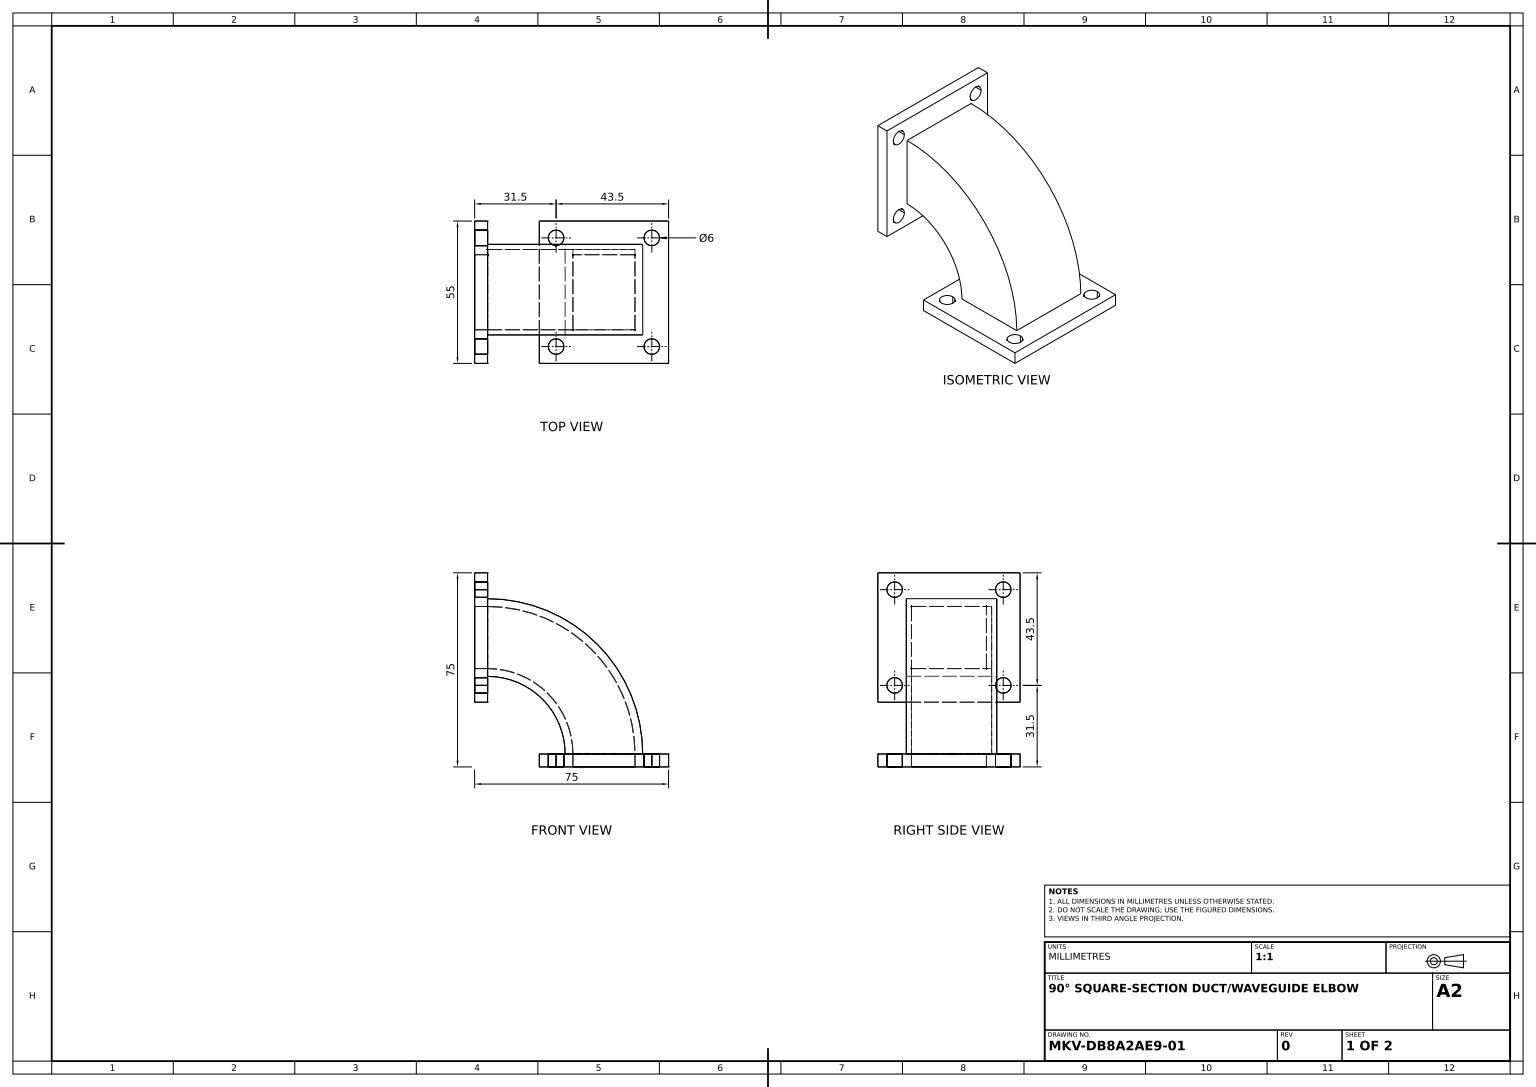
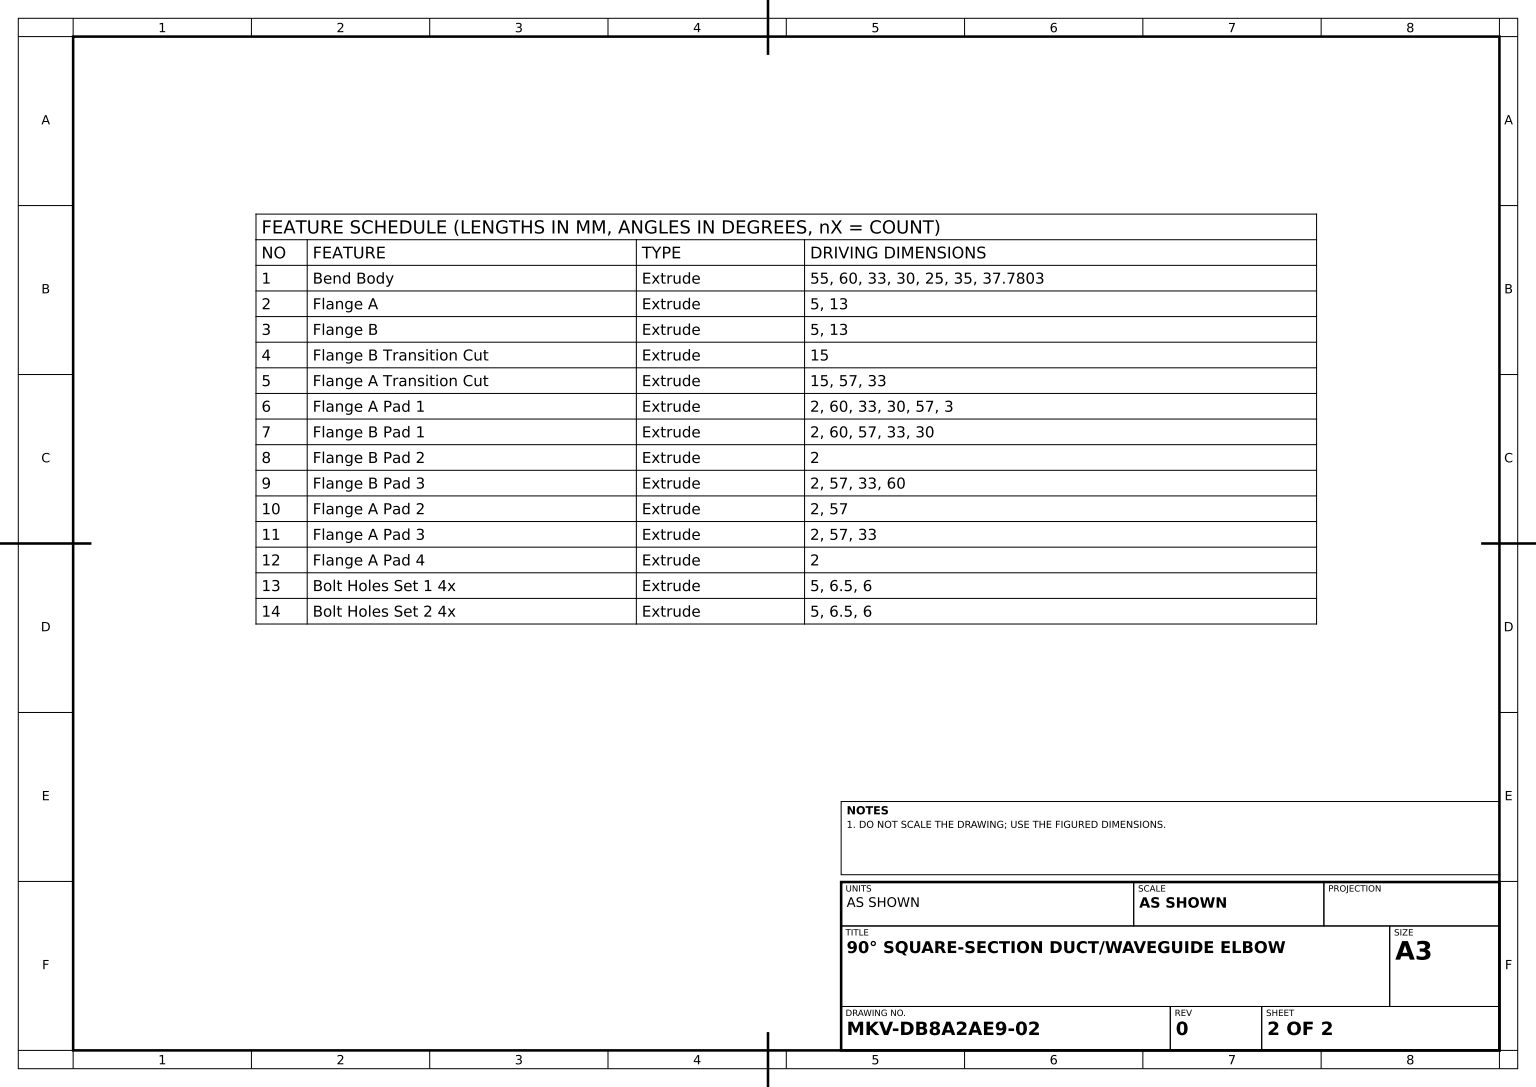
from build123d import *

# Parameters (mm, degrees)
BEND_BODY_DEPTH               = 55
BEND_BODY_2_DEPTH             = 55
FLANGE_A_SKETCH_W             = 24
FLANGE_A_SKETCH_H             = 13
FLANGE_A_DEPTH                = 5
FLANGE_B_SKETCH_W             = 13
FLANGE_B_SKETCH_H             = 24
FLANGE_B_DEPTH                = 5
FLANGE_START                  = -15
FLANGE_B_TRANSITION_CUT_DEPTH = 15
FLANGE_A_TRANSITION_CUT_DEPTH = 15
FLANGE_START_2                = 2
FLANGE_A_PAD_1_DEPTH          = 2
FLANGE_B_PAD_1_DEPTH          = 2
FLANGE_B_PAD_2_DEPTH          = 2
FLANGE_START_3                = -2
FLANGE_B_PAD_3_DEPTH          = 2
FLANGE_A_PAD_2_DEPTH          = 2
FLANGE_A_PAD_3_DEPTH          = 2
FLANGE_A_PAD_4_DEPTH          = 2
BOLT_HOLES_SET_1_SKETCH_R     = 3
BOLT_HOLES_SET_1_4X_DEPTH     = 5
BOLT_HOLES_SET_2_SKETCH_R     = 3
BOLT_HOLES_SET_2_4X_DEPTH     = 5


with BuildPart() as part:
    # Bend Profile Sketch → Bend Body (new body)
    with BuildSketch(Plane.XY):
        with BuildLine():
            Line((0, 57), (-5, 57))
            Line((-5, 57), (-5, 70))
            Line((-5, 70), (0, 70))
            Line((0, 70), (0, 60))
            ThreePointArc((0, 60), (42.426406871, 42.426406871), (60, 0))
            Line((60, 0), (70, 0))
            Line((70, 0), (70, -5))
            Line((70, -5), (57, -5))
            Line((57, -5), (57, 0))
            ThreePointArc((57, 0), (40.305086528, 40.305086528), (0, 57))
        make_face()
    extrude(amount=BEND_BODY_DEPTH)



with BuildPart() as body_2:
    # Bend Profile Sketch → Bend Body 2 (new body)
    with BuildSketch(Plane.XY):
        with BuildLine():
            Line((0, 33), (-5, 33))
            Line((-5, 33), (-5, 20))
            Line((-5, 20), (0, 20))
            Line((0, 20), (0, 30))
            ThreePointArc((0, 30), (21.213203436, 21.213203436), (30, 0))
            Line((30, 0), (20, 0))
            Line((20, 0), (20, -5))
            Line((20, -5), (33, -5))
            Line((33, -5), (33, 0))
            ThreePointArc((33, 0), (23.334523779, 23.334523779), (0, 33))
        make_face()
    extrude(amount=BEND_BODY_2_DEPTH)


with BuildPart() as part_1:
    add(part.part)

    add(body_2.part)  # Flange A merges body 2
    # Flange A Sketch → Flange A (add)
    with BuildSketch(Plane(origin=(0, -5, 0), x_dir=(-1, 0, 0), z_dir=(0, -1, 0))):
        with Locations((-45, -48.5)):
            Rectangle(FLANGE_A_SKETCH_W, FLANGE_A_SKETCH_H)
        with Locations((-45, -6.5)):
            Rectangle(FLANGE_A_SKETCH_W, FLANGE_A_SKETCH_H)
    extrude(amount=-FLANGE_A_DEPTH)

    # Flange B Sketch → Flange B (add)
    with BuildSketch(Plane.ZY.offset(5)):
        with Locations((48.5, 45)):
            Rectangle(FLANGE_B_SKETCH_W, FLANGE_B_SKETCH_H)
        with Locations((6.5, 45)):
            Rectangle(FLANGE_B_SKETCH_W, FLANGE_B_SKETCH_H)
    extrude(amount=-FLANGE_B_DEPTH)

    # Flange B Transition Cut Sketch → Flange B Transition Cut (cut)
    with BuildSketch(Plane.XY.offset(55).offset(FLANGE_START)):
        with BuildLine():
            Line((57, 0), (60, 0))
            ThreePointArc((60, 0), (42.426406871, 42.426406871), (0, 60))
            Line((0, 60), (0, 57))
            ThreePointArc((0, 57), (40.305086528, 40.305086528), (57, 0))
        make_face()
        with BuildLine():
            Line((30, 0), (33, 0))
            ThreePointArc((33, 0), (23.334523779, 23.334523779), (0, 33))
            Line((0, 33), (0, 30))
            ThreePointArc((0, 30), (21.213203436, 21.213203436), (30, 0))
        make_face()
    extrude(amount=FLANGE_B_TRANSITION_CUT_DEPTH, mode=Mode.SUBTRACT)

    # Flange A Transition Cut Sketch → Flange A Transition Cut (cut)
    with BuildSketch(Plane(origin=(0, 0, 0), x_dir=(-1, 0, 0), z_dir=(0, 0, -1))):
        with BuildLine():
            Line((0, 57), (0, 60))
            ThreePointArc((0, 60), (-42.426406871, 42.426406871), (-60, 0))
            Line((-60, 0), (-57, 0))
            ThreePointArc((-57, 0), (-40.305086528, 40.305086528), (0, 57))
        make_face()
        with BuildLine():
            Line((0, 30), (0, 33))
            ThreePointArc((0, 33), (-23.334523779, 23.334523779), (-33, 0))
            Line((-33, 0), (-30, 0))
            ThreePointArc((-30, 0), (-21.213203436, 21.213203436), (0, 30))
        make_face()
    extrude(amount=-FLANGE_A_TRANSITION_CUT_DEPTH, mode=Mode.SUBTRACT)

    # Flange A Pad 1 Sketch → Flange A Pad 1 (add)
    with BuildSketch(Plane(origin=(0, 0, 15), x_dir=(-1, 0, 0), z_dir=(0, 0, -1)).offset(FLANGE_START_2)):
        with BuildLine():
            Line((0, 60), (0, 57))
            ThreePointArc((0, 57), (-40.305086528, 40.305086528), (-57, 0))
            Line((-57, 0), (-60, 0))
            ThreePointArc((-60, 0), (-42.426406871, 42.426406871), (0, 60))
        make_face()
        with BuildLine():
            Line((-33, 0), (-30, 0))
            ThreePointArc((-30, 0), (-21.213203436, 21.213203436), (0, 30))
            Line((0, 30), (0, 33))
            ThreePointArc((0, 33), (-23.334523779, 23.334523779), (-33, 0))
        make_face()
    extrude(amount=-FLANGE_A_PAD_1_DEPTH)

    # Flange B Pad 1 Sketch → Flange B Pad 1 (add)
    with BuildSketch(Plane.XY.offset(40)):
        with BuildLine():
            Line((0, 60), (0, 57))
            ThreePointArc((0, 57), (40.305086528, 40.305086528), (57, 0))
            Line((57, 0), (60, 0))
            ThreePointArc((60, 0), (42.426406871, 42.426406871), (0, 60))
        make_face()
        with BuildLine():
            Line((30, 0), (33, 0))
            ThreePointArc((33, 0), (23.334523779, 23.334523779), (0, 33))
            Line((0, 33), (0, 30))
            ThreePointArc((0, 30), (21.213203436, 21.213203436), (30, 0))
        make_face()
    extrude(amount=FLANGE_B_PAD_1_DEPTH)

    # Flange B Pad 2 Sketch → Flange B Pad 2 (add)
    with BuildSketch(Plane.XY.offset(42)):
        with BuildLine():
            Line((0, 60), (0, 57))
            ThreePointArc((0, 57), (40.305086528, 40.305086528), (57, 0))
            Line((57, 0), (60, 0))
            ThreePointArc((60, 0), (42.426406871, 42.426406871), (0, 60))
        make_face()
        with BuildLine():
            ThreePointArc((33, 0), (23.334523779, 23.334523779), (0, 33))
            Line((0, 33), (0, 30))
            ThreePointArc((0, 30), (21.213203436, 21.213203436), (30, 0))
            Line((30, 0), (33, 0))
        make_face()
    extrude(amount=FLANGE_B_PAD_2_DEPTH)

    # Flange B Pad 3 Sketch → Flange B Pad 3 (add)
    with BuildSketch(Plane.XY.offset(44).offset(FLANGE_START_3)):
        with BuildLine():
            ThreePointArc((57, 0), (40.305086528, 40.305086528), (0, 57))
            Line((0, 57), (0, 33))
            ThreePointArc((0, 33), (23.334523779, 23.334523779), (33, 0))
            Line((33, 0), (57, 0))
        make_face()
    extrude(amount=FLANGE_B_PAD_3_DEPTH)

    # Flange A Pad 2 Sketch → Flange A Pad 2 (add)
    with BuildSketch(Plane(origin=(0, 0, 13), x_dir=(-1, 0, 0), z_dir=(0, 0, -1)).offset(FLANGE_START_2)):
        with BuildLine():
            Line((0, 57), (0, 60))
            ThreePointArc((0, 60), (-42.426406871, 42.426406871), (-60, 0))
            Line((-60, 0), (-57, 0))
            ThreePointArc((-57, 0), (-40.305086528, 40.305086528), (0, 57))
        make_face()
        with BuildLine():
            Line((0, 30), (0, 33))
            ThreePointArc((0, 33), (-23.334523779, 23.334523779), (-33, 0))
            Line((-33, 0), (-30, 0))
            ThreePointArc((-30, 0), (-21.213203436, 21.213203436), (0, 30))
        make_face()
    extrude(amount=-FLANGE_A_PAD_2_DEPTH)

    # Flange A Pad 3 Sketch → Flange A Pad 3 (add)
    with BuildSketch(Plane(origin=(0, 0, 11), x_dir=(-1, 0, 0), z_dir=(0, 0, -1)).offset(FLANGE_START_2)):
        with BuildLine():
            Line((0, 57), (0, 60))
            ThreePointArc((0, 60), (-42.426406871, 42.426406871), (-60, 0))
            Line((-60, 0), (-57, 0))
            ThreePointArc((-57, 0), (-40.305086528, 40.305086528), (0, 57))
        make_face()
        with BuildLine():
            Line((0, 30), (0, 33))
            ThreePointArc((0, 33), (-23.334523779, 23.334523779), (-33, 0))
            Line((-33, 0), (-30, 0))
            ThreePointArc((-30, 0), (-21.213203436, 21.213203436), (0, 30))
        make_face()
    extrude(amount=-FLANGE_A_PAD_3_DEPTH)

    # Flange A Pad 4 Sketch → Flange A Pad 4 (add)
    with BuildSketch(Plane(origin=(0, 0, 9), x_dir=(-1, 0, 0), z_dir=(0, 0, -1))):
        with BuildLine():
            Line((-57, 0), (-33, 0))
            ThreePointArc((-33, 0), (-23.334523779, 23.334523779), (0, 33))
            Line((0, 33), (0, 57))
            ThreePointArc((0, 57), (-40.305086528, 40.305086528), (-57, 0))
        make_face()
    extrude(amount=-FLANGE_A_PAD_4_DEPTH)

    # Bolt Holes Set 1 Sketch → Bolt Holes Set 1 4x (cut)
    with BuildSketch(Plane.ZY.offset(5)):
        with Locations((6.5, 63.5)):
            Circle(BOLT_HOLES_SET_1_SKETCH_R)
        with Locations((48.5, 63.5)):
            Circle(BOLT_HOLES_SET_1_SKETCH_R)
        with Locations((48.5, 26.5)):
            Circle(BOLT_HOLES_SET_1_SKETCH_R)
        with Locations((6.5, 26.5)):
            Circle(BOLT_HOLES_SET_1_SKETCH_R)
    extrude(amount=-BOLT_HOLES_SET_1_4X_DEPTH, mode=Mode.SUBTRACT)

    # Bolt Holes Set 2 Sketch → Bolt Holes Set 2 4x (cut)
    with BuildSketch(Plane.XZ.offset(5)):
        with Locations(Location((26.5, 48.5, 0), (0, 0, 270))):
            Circle(BOLT_HOLES_SET_2_SKETCH_R)
        with Locations(Location((63.5, 48.5, 0), (0, 0, 270))):
            Circle(BOLT_HOLES_SET_2_SKETCH_R)
        with Locations(Location((63.5, 6.5, 0), (0, 0, 270))):
            Circle(BOLT_HOLES_SET_2_SKETCH_R)
        with Locations(Location((26.5, 6.5, 0), (0, 0, 270))):
            Circle(BOLT_HOLES_SET_2_SKETCH_R)
    extrude(amount=-BOLT_HOLES_SET_2_4X_DEPTH, mode=Mode.SUBTRACT)


solid = part_1.part
